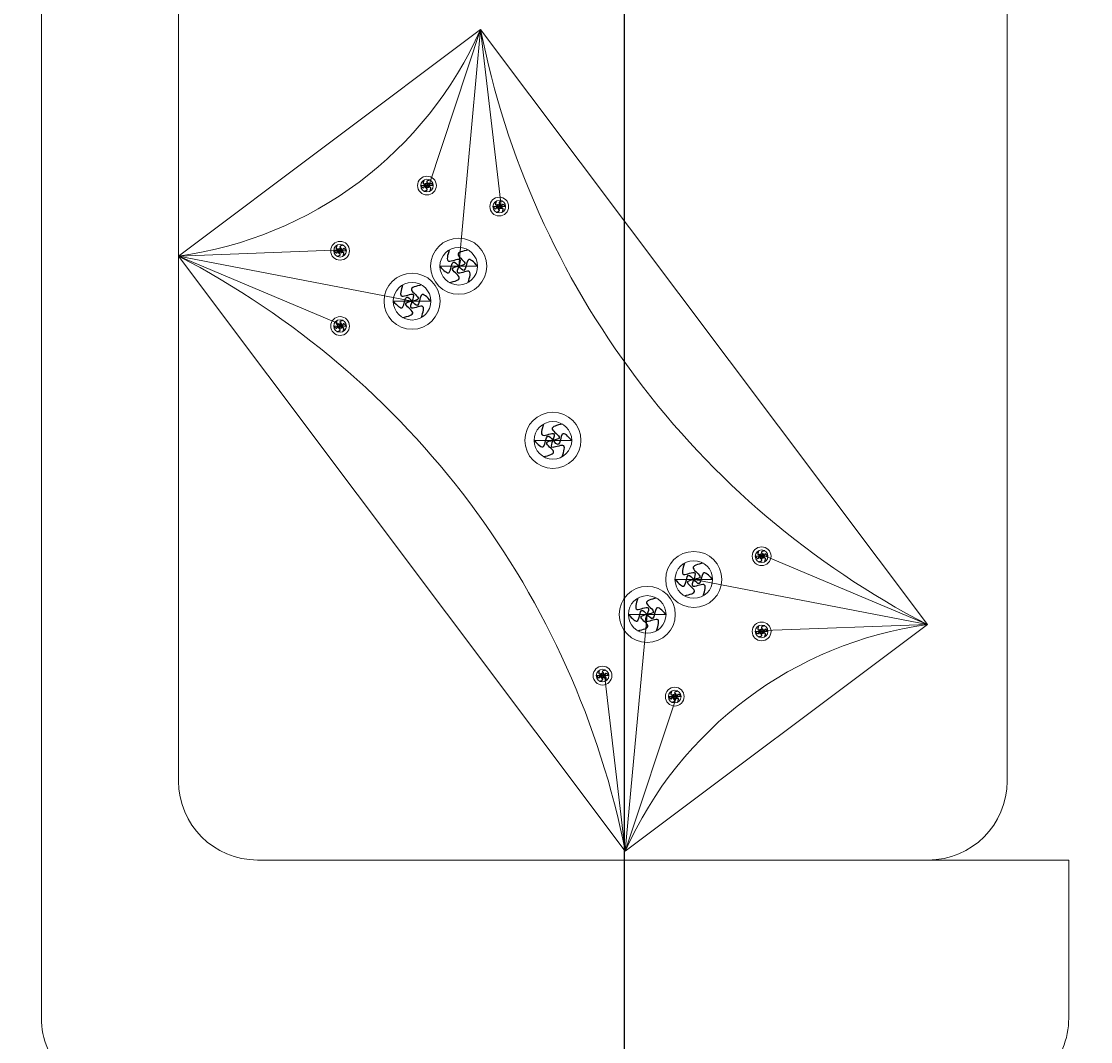
# Model space of a CAD drawing. Units: inches. Extents: x -61 to 1599, y -1316 to 257.
# Tile 25 of 204: x 388 to 416, y -912 to -886. Entities that reach past the tile are written whole.
import ezdxf

# ---------------------------------------------------------------- set-up
doc = ezdxf.new("R2010")
doc.units = ezdxf.units.IN
doc.header["$MEASUREMENT"] = 0
doc.layers.add('A-ANNO-DIMS', color=2, linetype='Continuous', lineweight=18)
doc.layers.add('FURNITURE', color=83, linetype='Continuous', lineweight=18)
doc.layers.add('FUR', color=83, linetype='Continuous')
doc.styles.get("Standard").update_dxf_attribs({"font": 'arial.ttf'})
doc.dimstyles.get("Standard").update_dxf_attribs({"dimtxt": 0.18, "dimasz": 0.18, "dimexe": 0.18, "dimexo": 0.0625, "dimgap": 0.09, "dimtad": 0, "dimtih": 1, "dimtoh": 1, "dimdec": 0, "dimzin": 0, "dimdsep": 46, "dimlunit": 3, "dimtxsty": 'Standard', "dimcen": 0.09, "dimadec": 0, "dimazin": 0, "dimtfac": 1, "dimtdec": 0, "dimtofl": 0, "dimtmove": 0, "dimatfit": 3, "dimfxl": 1, "dimtolj": 1, "dimtzin": 0, "dimarcsym": 0})

# ---------------------------------------------------------------- blocks, each defined once
blk = doc.blocks.new('*U160')
at = {"layer": 'FUR'}
blk.add_open_spline([(0.005, 0.08), (-0.03, 0.048), (-0.098, -0.015), (0.075, -0.018), (0.024, -0.063), (0.005, -0.08)], degree=3, knots=[0, 0, 0, 0, 0.0954578, 0.1898773, 0.2470677, 0.2470677, 0.2470677, 0.2470677], dxfattribs=at)
blk = doc.blocks.new('*U161')
at = {"layer": 'FUR', "transparency": 16777216}
for p, rotation in [((222.173, -79.977), 60), ((222.178, -80.056), 120), ((222.25, -80.092), 180), ((222.312, -79.968), 300), ((222.317, -80.048), 240)]:
    blk.add_blockref('*U160', p, dxfattribs=dict(at, rotation=rotation))
blk.add_blockref('*U160', (222.24, -79.932), dxfattribs=at)
blk = doc.blocks.new('*U172')
at = {"layer": 'FUR'}
blk.add_open_spline([(0.005, 0.08), (-0.03, 0.048), (-0.098, -0.015), (0.075, -0.018), (0.024, -0.063), (0.005, -0.08)], degree=3, knots=[0, 0, 0, 0, 0.0954578, 0.1898773, 0.2470677, 0.2470677, 0.2470677, 0.2470677], dxfattribs=at)
blk = doc.blocks.new('*U173')
at = {"layer": 'FUR', "transparency": 16777216}
for p, rotation in [((222.173, -79.977), 60), ((222.178, -80.056), 120), ((222.25, -80.092), 180), ((222.312, -79.968), 300), ((222.317, -80.048), 240)]:
    blk.add_blockref('*U172', p, dxfattribs=dict(at, rotation=rotation))
blk.add_blockref('*U172', (222.24, -79.932), dxfattribs=at)
blk = doc.blocks.new('*U184')
at = {"layer": 'FUR'}
blk.add_open_spline([(0.015, 0.238), (-0.088, 0.143), (-0.292, -0.045), (0.224, -0.053), (0.072, -0.187), (0.015, -0.238)], degree=3, knots=[0, 0, 0, 0, 0.2846533, 0.5662105, 0.736751, 0.736751, 0.736751, 0.736751], dxfattribs=at)
blk = doc.blocks.new('*U159')
at = {"layer": 'FUR', "transparency": 16777216}
blk.add_blockref('*U184', (662.716, -238.357), dxfattribs=at)
for p, rotation in [((662.517, -238.489), 60), ((662.929, -238.463), 300), ((662.531, -238.727), 120), ((662.745, -238.833), 180), ((662.944, -238.702), 240)]:
    blk.add_blockref('*U184', p, dxfattribs=dict(at, rotation=rotation))
blk = doc.blocks.new('*U174')
at = {"layer": 'FUR'}
blk.add_open_spline([(0.005, 0.08), (-0.03, 0.048), (-0.098, -0.015), (0.075, -0.018), (0.024, -0.063), (0.005, -0.08)], degree=3, knots=[0, 0, 0, 0, 0.0954578, 0.1898773, 0.2470677, 0.2470677, 0.2470677, 0.2470677], dxfattribs=at)
blk = doc.blocks.new('*U175')
at = {"layer": 'FUR', "transparency": 16777216}
for p, rotation in [((222.173, -79.977), 60), ((222.178, -80.056), 120), ((222.25, -80.092), 180), ((222.312, -79.968), 300), ((222.317, -80.048), 240)]:
    blk.add_blockref('*U174', p, dxfattribs=dict(at, rotation=rotation))
blk.add_blockref('*U174', (222.24, -79.932), dxfattribs=at)
blk = doc.blocks.new('*U168')
at = {"layer": 'FUR'}
blk.add_open_spline([(0.015, 0.238), (-0.088, 0.143), (-0.292, -0.045), (0.224, -0.053), (0.072, -0.187), (0.015, -0.238)], degree=3, knots=[0, 0, 0, 0, 0.2846533, 0.5662105, 0.736751, 0.736751, 0.736751, 0.736751], dxfattribs=at)
blk = doc.blocks.new('*U169')
at = {"layer": 'FUR', "transparency": 16777216}
blk.add_blockref('*U168', (662.716, -238.357), dxfattribs=at)
for p, rotation in [((662.517, -238.489), 60), ((662.929, -238.463), 300), ((662.531, -238.727), 120), ((662.745, -238.833), 180), ((662.944, -238.702), 240)]:
    blk.add_blockref('*U168', p, dxfattribs=dict(at, rotation=rotation))
blk = doc.blocks.new('*U176')
at = {"layer": 'FUR'}
blk.add_open_spline([(0.005, 0.08), (-0.03, 0.048), (-0.098, -0.015), (0.075, -0.018), (0.024, -0.063), (0.005, -0.08)], degree=3, knots=[0, 0, 0, 0, 0.0954578, 0.1898773, 0.2470677, 0.2470677, 0.2470677, 0.2470677], dxfattribs=at)
blk = doc.blocks.new('*U177')
at = {"layer": 'FUR', "transparency": 16777216}
for p, rotation in [((222.173, -79.977), 60), ((222.178, -80.056), 120), ((222.25, -80.092), 180), ((222.312, -79.968), 300), ((222.317, -80.048), 240)]:
    blk.add_blockref('*U176', p, dxfattribs=dict(at, rotation=rotation))
blk.add_blockref('*U176', (222.24, -79.932), dxfattribs=at)
blk = doc.blocks.new('*U170')
at = {"layer": 'FUR'}
blk.add_open_spline([(0.015, 0.238), (-0.088, 0.143), (-0.292, -0.045), (0.224, -0.053), (0.072, -0.187), (0.015, -0.238)], degree=3, knots=[0, 0, 0, 0, 0.2846533, 0.5662105, 0.736751, 0.736751, 0.736751, 0.736751], dxfattribs=at)
blk = doc.blocks.new('*U171')
at = {"layer": 'FUR', "transparency": 16777216}
blk.add_blockref('*U170', (662.716, -238.357), dxfattribs=at)
for p, rotation in [((662.517, -238.489), 60), ((662.929, -238.463), 300), ((662.531, -238.727), 120), ((662.745, -238.833), 180), ((662.944, -238.702), 240)]:
    blk.add_blockref('*U170', p, dxfattribs=dict(at, rotation=rotation))
blk = doc.blocks.new('*U164')
at = {"layer": 'FUR'}
blk.add_open_spline([(0.005, 0.08), (-0.03, 0.048), (-0.098, -0.015), (0.075, -0.018), (0.024, -0.063), (0.005, -0.08)], degree=3, knots=[0, 0, 0, 0, 0.0954578, 0.1898773, 0.2470677, 0.2470677, 0.2470677, 0.2470677], dxfattribs=at)
blk = doc.blocks.new('*U165')
at = {"layer": 'FUR', "transparency": 16777216}
for p, rotation in [((222.173, -79.977), 60), ((222.178, -80.056), 120), ((222.25, -80.092), 180), ((222.312, -79.968), 300), ((222.317, -80.048), 240)]:
    blk.add_blockref('*U164', p, dxfattribs=dict(at, rotation=rotation))
blk.add_blockref('*U164', (222.24, -79.932), dxfattribs=at)
blk = doc.blocks.new('*U183')
at = {"layer": 'FUR'}
blk.add_open_spline([(0.015, 0.238), (-0.088, 0.143), (-0.292, -0.045), (0.224, -0.053), (0.072, -0.187), (0.015, -0.238)], degree=3, knots=[0, 0, 0, 0, 0.2846533, 0.5662105, 0.736751, 0.736751, 0.736751, 0.736751], dxfattribs=at)
blk = doc.blocks.new('*U162')
at = {"layer": 'FUR', "transparency": 16777216}
blk.add_blockref('*U183', (662.716, -238.357), dxfattribs=at)
for p, rotation in [((662.517, -238.489), 60), ((662.929, -238.463), 300), ((662.531, -238.727), 120), ((662.745, -238.833), 180), ((662.944, -238.702), 240)]:
    blk.add_blockref('*U183', p, dxfattribs=dict(at, rotation=rotation))
blk = doc.blocks.new('*U182')
at = {"layer": 'FUR'}
blk.add_open_spline([(0.005, 0.08), (-0.03, 0.048), (-0.098, -0.015), (0.075, -0.018), (0.024, -0.063), (0.005, -0.08)], degree=3, knots=[0, 0, 0, 0, 0.0954578, 0.1898773, 0.2470677, 0.2470677, 0.2470677, 0.2470677], dxfattribs=at)
blk = doc.blocks.new('*U163')
at = {"layer": 'FUR', "transparency": 16777216}
for p, rotation in [((222.173, -79.977), 60), ((222.178, -80.056), 120), ((222.25, -80.092), 180), ((222.312, -79.968), 300), ((222.317, -80.048), 240)]:
    blk.add_blockref('*U182', p, dxfattribs=dict(at, rotation=rotation))
blk.add_blockref('*U182', (222.24, -79.932), dxfattribs=at)
blk = doc.blocks.new('*U166')
at = {"layer": 'FUR'}
blk.add_open_spline([(0.015, 0.238), (-0.088, 0.143), (-0.292, -0.045), (0.224, -0.053), (0.072, -0.187), (0.015, -0.238)], degree=3, knots=[0, 0, 0, 0, 0.2846533, 0.5662105, 0.736751, 0.736751, 0.736751, 0.736751], dxfattribs=at)
blk = doc.blocks.new('*U167')
at = {"layer": 'FUR', "transparency": 16777216}
blk.add_blockref('*U166', (662.716, -238.357), dxfattribs=at)
for p, rotation in [((662.517, -238.489), 60), ((662.929, -238.463), 300), ((662.531, -238.727), 120), ((662.745, -238.833), 180), ((662.944, -238.702), 240)]:
    blk.add_blockref('*U166', p, dxfattribs=dict(at, rotation=rotation))
blk = doc.blocks.new('*U178')
at = {"layer": 'FUR'}
blk.add_open_spline([(0.005, 0.08), (-0.03, 0.048), (-0.098, -0.015), (0.075, -0.018), (0.024, -0.063), (0.005, -0.08)], degree=3, knots=[0, 0, 0, 0, 0.0954578, 0.1898773, 0.2470677, 0.2470677, 0.2470677, 0.2470677], dxfattribs=at)
blk = doc.blocks.new('*U179')
at = {"layer": 'FUR', "transparency": 16777216}
for p, rotation in [((222.173, -79.977), 60), ((222.178, -80.056), 120), ((222.25, -80.092), 180), ((222.312, -79.968), 300), ((222.317, -80.048), 240)]:
    blk.add_blockref('*U178', p, dxfattribs=dict(at, rotation=rotation))
blk.add_blockref('*U178', (222.24, -79.932), dxfattribs=at)
blk = doc.blocks.new('*U180')
at = {"layer": 'FUR'}
blk.add_open_spline([(0.005, 0.08), (-0.03, 0.048), (-0.098, -0.015), (0.075, -0.018), (0.024, -0.063), (0.005, -0.08)], degree=3, knots=[0, 0, 0, 0, 0.0954578, 0.1898773, 0.2470677, 0.2470677, 0.2470677, 0.2470677], dxfattribs=at)
blk = doc.blocks.new('*U181')
at = {"layer": 'FUR', "transparency": 16777216}
for p, rotation in [((222.173, -79.977), 60), ((222.178, -80.056), 120), ((222.25, -80.092), 180), ((222.312, -79.968), 300), ((222.317, -80.048), 240)]:
    blk.add_blockref('*U180', p, dxfattribs=dict(at, rotation=rotation))
blk.add_blockref('*U180', (222.24, -79.932), dxfattribs=at)
blk = doc.blocks.new('SOFA-LOVESEAT')
for p, q in [((3.47, 8), (3.47, 52)), ((24.442, 8), (24.442, 28)), ((11.116, 27.026), (9.811, 23.092)), ((11.116, 27.026), (10.561, 21.032)), ((11.116, 27.026), (11.639, 22.56)), ((9.759, 23.073), (9.599, 23.073)), ((9.759, 23.073), (9.918, 23.073)), ((11.587, 22.541), (11.427, 22.541)), ((11.587, 22.541), (11.747, 22.541)), ((3.47, 21.288), (7.612, 21.442)), ((7.56, 21.423), (7.4, 21.423)), ((7.56, 21.423), (7.719, 21.423)), ((3.47, 21.288), (9.381, 20.146)), ((3.47, 21.288), (7.612, 19.538)), ((10.561, 21.032), (10.084, 21.032)), ((10.561, 21.032), (11.037, 21.032)), ((9.381, 20.146), (8.904, 20.146)), ((9.381, 20.146), (9.857, 20.146)), ((7.56, 19.518), (7.4, 19.518)), ((7.56, 19.518), (7.719, 19.518)), ((12.946, 16.624), (12.47, 16.624)), ((12.946, 16.624), (13.423, 16.624)), ((18.228, 13.691), (18.068, 13.691)), ((18.228, 13.691), (18.388, 13.691)), ((22.422, 11.961), (18.28, 13.711)), ((16.511, 13.102), (16.035, 13.102)), ((22.422, 11.961), (16.511, 13.102)), ((16.511, 13.102), (16.988, 13.102)), ((14.776, 6.223), (15.332, 12.217)), ((15.332, 12.217), (14.855, 12.217)), ((15.332, 12.217), (15.808, 12.217)), ((22.422, 11.961), (18.28, 11.807)), ((18.228, 11.787), (18.068, 11.787)), ((18.228, 11.787), (18.388, 11.787)), ((14.201, 10.669), (14.041, 10.669)), ((14.201, 10.669), (14.36, 10.669)), ((14.776, 6.223), (14.253, 10.689)), ((14.776, 6.223), (16.081, 10.156)), ((16.029, 10.137), (15.869, 10.137)), ((16.029, 10.137), (16.189, 10.137)), ((22.442, 6), (5.47, 6)), ((22.442, 6), (26, 6))]:
    blk.add_line(p, q)
blk.add_lwpolyline([(26, 6), (26, 2, -0.414214), (24, 0), (2, 0, -0.414214), (0, 2), (0, 58, -0.414213), (2, 60), (24, 60, -0.414214), (26, 58), (26, 54)], format="xyb")
blk.add_lwpolyline([(11.116, 27.026), (22.422, 11.961), (14.776, 6.223), (3.47, 21.288)], close=True)
for centre, radius in [((9.759, 23.073), 0.238), ((9.759, 23.073), 0.16), ((11.587, 22.541), 0.238), ((11.587, 22.541), 0.16), ((7.56, 21.423), 0.238), ((10.561, 21.032), 0.71), ((7.56, 21.423), 0.16), ((10.561, 21.032), 0.476), ((9.381, 20.146), 0.71), ((9.381, 20.146), 0.476), ((7.56, 19.518), 0.238), ((7.56, 19.518), 0.16), ((12.946, 16.624), 0.71), ((12.946, 16.624), 0.476), ((16.511, 13.102), 0.71), ((18.228, 13.691), 0.238), ((18.228, 13.691), 0.16), ((16.511, 13.102), 0.476), ((15.332, 12.217), 0.71), ((15.332, 12.217), 0.476), ((18.228, 11.787), 0.238), ((18.228, 11.787), 0.16), ((14.201, 10.669), 0.238), ((14.201, 10.669), 0.16), ((16.029, 10.137), 0.238), ((16.029, 10.137), 0.16)]:
    blk.add_circle(centre, radius)
for centre, radius, start, end in [((2.147, 31.014), 9.816, 277.747, 336.0258), ((32.433, 31.248), 21.731, 191.2044, 242.5684), ((-6.541, 2), 21.731, 11.2044, 62.5684), ((23.745, 2.234), 9.816, 97.747, 156.0258), ((5.47, 8), 2, 180, 270), ((22.442, 8), 2, 270, 0)]:
    blk.add_arc(centre, radius, start, end)
at = {"rotation": 90}
for name, p in [('*U175', (-70.254, -199.172)), ('*U177', (-68.425, -199.704)), ('*U173', (-72.453, -200.822)), ('*U169', (-228.034, -641.698)), ('*U159', (-229.214, -642.584)), ('*U161', (-72.453, -202.727)), ('*U171', (-225.649, -646.106)), ('*U181', (-61.785, -208.554)), ('*U167', (-222.084, -649.628)), ('*U162', (-223.264, -650.513)), ('*U179', (-61.785, -210.458)), ('*U165', (-65.812, -211.576)), ('*U163', (-63.983, -212.108))]:
    blk.add_blockref(name, p, dxfattribs=at)
blk = doc.blocks.new('*D696')
at = {"layer": 'A-ANNO-DIMS', "color": 0, "lineweight": -2, "transparency": 16777216}
for p, q in [((690.64, -873.169), (-61.077, -873.169)), ((-60.897, -873.349), (-60.897, -1025.799)), ((-60.897, -1178.613), (-60.897, -1026.163)), ((690.64, -1178.793), (-61.077, -1178.793))]:
    blk.add_line(p, q, dxfattribs=at)
at = {"layer": 'A-ANNO-DIMS', "color": 0, "transparency": 16777216}
for points in [[(-60.927, -873.349), (-60.867, -873.349), (-60.897, -873.169)], [(-60.927, -1178.613), (-60.867, -1178.613), (-60.897, -1178.793)]]:
    blk.add_solid(points, dxfattribs=at)
at = {"layer": 'DEFPOINTS', "color": 0, "transparency": 16777216}
for p in [(-60.897, -873.169), (690.703, -873.169), (690.703, -1178.793)]:
    blk.add_point(p, dxfattribs=at)
at = {"layer": 'A-ANNO-DIMS', "color": 0, "transparency": 16777216, "insert": (-60.897, -1025.981), "char_height": 0.18, "attachment_point": 5}
blk.add_mtext('\\A1;305.6', dxfattribs=at)
blk = doc.blocks.new('*D710')
at = {"layer": 'A-ANNO-DIMS', "color": 0, "lineweight": -2, "transparency": 16777216}
for p, q in [((319.703, -465.385), (319.703, -1315.725)), ((403.703, -465.385), (403.703, -1315.725)), ((319.883, -1315.545), (361.484, -1315.545)), ((403.523, -1315.545), (361.921, -1315.545))]:
    blk.add_line(p, q, dxfattribs=at)
at = {"layer": 'A-ANNO-DIMS', "color": 0, "transparency": 16777216}
for points in [[(319.883, -1315.515), (319.883, -1315.575), (319.703, -1315.545)], [(403.523, -1315.515), (403.523, -1315.575), (403.703, -1315.545)]]:
    blk.add_solid(points, dxfattribs=at)
at = {"layer": 'DEFPOINTS', "color": 0, "transparency": 16777216}
for p in [(319.703, -465.323), (403.703, -465.323), (403.703, -1315.545)]:
    blk.add_point(p, dxfattribs=at)
at = {"layer": 'A-ANNO-DIMS', "color": 0, "transparency": 16777216, "insert": (361.703, -1315.545), "char_height": 0.18, "attachment_point": 5}
blk.add_mtext('\\A1;84', dxfattribs=at)

msp = doc.modelspace()

# ---------------------------------------------------------------- block references
at = {"layer": 'FURNITURE'}
msp.add_blockref('SOFA-LOVESEAT', (388.9518, -913.0047), dxfattribs=at)

# ---------------------------------------------------------------- dimensions: what is measured, and where the dimension line sits
at = {"layer": 'A-ANNO-DIMS'}
dim = msp.add_linear_dim(base=(403.7028, -1315.5446), p1=(319.7028, -465.3229), p2=(403.7028, -465.3229), dimstyle='Standard', override={"dimdec": 0, "dimlfac": 1, "dimrnd": 0, "dimzin": 0, "dimdsep": 46, "dimlunit": 2}, dxfattribs=at)
dim.commit()
dim.dimension.update_dxf_attribs({"geometry": '*D710', "text_midpoint": (361.7028, -1315.5446)})
dim = msp.add_linear_dim(base=(-60.8972, -873.169), p1=(690.7028, -1178.7933), p2=(690.7028, -873.169), angle=90, dimstyle='Standard', override={"dimdec": 1, "dimlfac": 1, "dimrnd": 0, "dimzin": 0, "dimdsep": 46, "dimlunit": 2}, dxfattribs=at)
dim.commit()
dim.dimension.update_dxf_attribs({"geometry": '*D696', "text_midpoint": (-60.8972, -1025.9812)})

doc.saveas('drawing.dxf')
